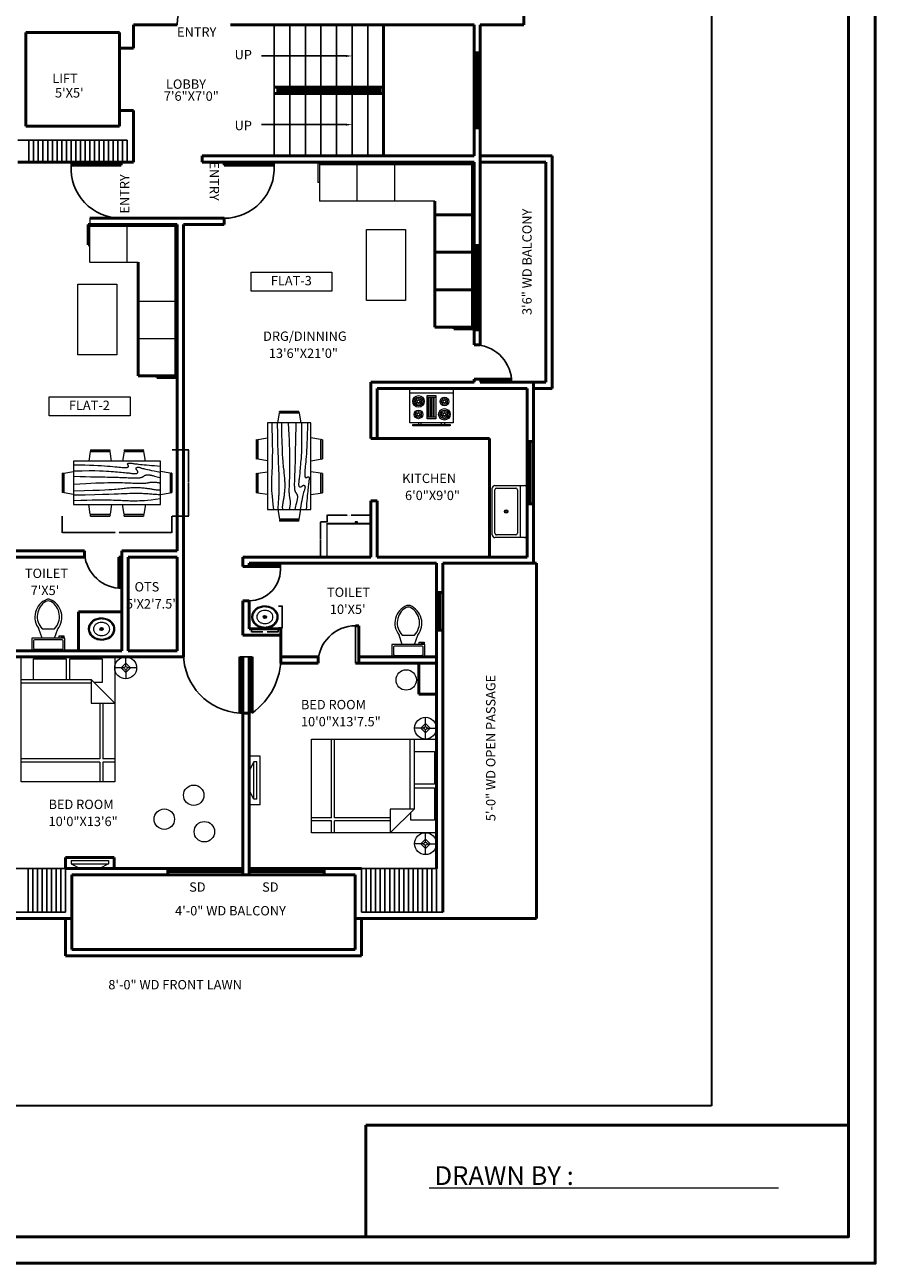
# Model space of a CAD drawing. Units: inches. Extents: x 1493 to 2377, y 814 to 2191.
# Tile 2 of 4: x 1832 to 2377, y 814 to 1607. Entities that reach past the tile are written whole.
import ezdxf
from ezdxf import colors
from ezdxf.entities.mleader import LeaderData, LeaderLine
from ezdxf.math import Vec2, Vec3

# ---------------------------------------------------------------- set-up
doc = ezdxf.new("R2010")
doc.units = ezdxf.units.IN
for name, color, linetype, lineweight in [('A-ANNO-DIMS', 2, 'Continuous', 18), ('A-ANNO-SYMB', 2, 'Continuous', 18), ('A-ANNO-TEXT', 3, 'Continuous', 18), ('A-ANNO-TTLB', 7, 'Continuous', 35), ('A-AREA-IDEN', 7, 'Continuous', 18), ('A-DOOR', 4, 'Continuous', 25), ('A-EQPM', 9, 'Continuous', 18), ('A-FLOR-FIXT', 8, 'Continuous', 18), ('A-FLOR-STRS', 3, 'Continuous', 25), ('A-FURN', 8, 'Continuous', 18), ('A-GLAZ', 4, 'Continuous', 25), ('A-WALL', 7, 'Continuous', 50)]:
    doc.layers.add(name, color=color, linetype=linetype, lineweight=lineweight)
doc.styles.get("Standard").update_dxf_attribs({"font": 'arial.ttf'})
doc.dimstyles.get("Standard").update_dxf_attribs({"dimtxt": 0.18, "dimasz": 0.18, "dimexe": 0.18, "dimexo": 0.0625, "dimgap": 0.09, "dimtad": 0, "dimtih": 1, "dimtoh": 1, "dimdec": 4, "dimzin": 0, "dimdsep": 46, "dimtxsty": 'Standard', "dimcen": 0.09, "dimadec": 0, "dimazin": 0, "dimtfac": 1, "dimtdec": 4, "dimtofl": 0, "dimtmove": 0, "dimatfit": 3, "dimfxl": 1, "dimtolj": 1, "dimtzin": 0, "dimarcsym": 0})

# ---------------------------------------------------------------- blocks, each defined once
blk = doc.blocks.new('Dining Set - 36 x 72 in.')
for p, q in [((-22.2343, 26.00059), (-23.4847, 17.99762)), ((-22.2304, 26), (-5.7608, 26)), ((-22, 27.5), (-22.1562, 26.50042)), ((-5.8416, 26.5), (-22.1534, 26.5)), ((-22, 27.5), (-6, 27.5)), ((-5.8437, 26.49966), (-6, 27.5)), ((-4.5152, 17.99762), (-5.7655, 25.99926)), ((5.7657, 26.00059), (4.5153, 17.99762)), ((5.7696, 26), (22.2392, 26)), ((6, 27.5), (5.8438, 26.50042)), ((22.1584, 26.5), (5.8466, 26.5)), ((6, 27.5), (22, 27.5)), ((22.1563, 26.49966), (22, 27.5)), ((23.4848, 17.99762), (22.2345, 25.99926)), ((36, 18), (-36, 18)), ((-36, 18), (-36, -18)), ((36, -18), (36, 18)), ((-45.5, 8), (-44.5004, 8.15617)), ((-45.5, 8), (-45.5, -8)), ((-44.5, -8.15843), (-44.5, 8.15338)), ((-44.0006, 8.23428), (-35.9976, 9.48474)), ((-44, 8.23041), (-44, -8.23915)), ((44.0006, 8.23428), (35.9976, 9.48474)), ((44, 8.23041), (44, -8.23915)), ((44.5, -8.15843), (44.5, 8.15338)), ((45.5, 8), (44.5005, 8.15617)), ((45.5, 8), (45.5, -8)), ((-44.4997, -8.15631), (-45.5, -8)), ((-35.9976, -9.48476), (-43.9993, -8.2345)), ((35.9976, -9.48476), (43.9993, -8.2345)), ((44.4997, -8.15631), (45.5, -8)), ((-36, -18), (36, -18)), ((-22.2343, -26.0006), (-23.4847, -17.99762)), ((-4.5152, -17.99762), (-5.7655, -25.99928)), ((5.7657, -26.0006), (4.5153, -17.99762)), ((23.4848, -17.99762), (22.2345, -25.99928)), ((-22.2304, -26), (-5.7608, -26)), ((-22, -27.5), (-22.1562, -26.50044)), ((-5.8416, -26.5), (-22.1534, -26.5)), ((-22, -27.5), (-6, -27.5)), ((-5.8437, -26.49967), (-6, -27.5)), ((5.7696, -26), (22.2392, -26)), ((6, -27.5), (5.8438, -26.50044)), ((22.1584, -26.5), (5.8466, -26.5)), ((6, -27.5), (22, -27.5)), ((22.1563, -26.49967), (22, -27.5))]:
    blk.add_line(p, q)
for points in [[(-36, 15), (-31.1772, 14.97754), (-26.8079, 14.91406), (-22.8538, 14.81543), (-19.276, 14.6875), (-16.0362, 14.53613), (-13.0957, 14.36718), (-10.4159, 14.18652), (-7.9583, 14), (-5.6904, 13.81315), (-3.6035, 13.63021), (-1.6954, 13.45508), (0.0365, 13.29166), (1.5945, 13.14388), (2.9811, 13.01562), (4.1988, 12.9108), (5.25, 12.83333), (6.1393, 12.78613), (6.8802, 12.76823), (7.4883, 12.77767), (7.9792, 12.8125), (8.3685, 12.87077), (8.6719, 12.95052), (8.9049, 13.0498), (9.0833, 13.16666), (9.2205, 13.29899), (9.3216, 13.44401), (9.3895, 13.59879), (9.4271, 13.76041), (9.4373, 13.92594), (9.4232, 14.09245), (9.3875, 14.257), (9.3333, 14.41666), (9.2638, 14.56917), (9.1836, 14.71484), (9.0975, 14.85465), (9.0104, 14.98958), (8.9272, 15.1206), (8.8529, 15.2487), (8.7922, 15.37483), (8.75, 15.5), (8.7305, 15.62467), (8.7344, 15.74739), (8.7617, 15.86621), (8.8125, 15.97916), (8.8867, 16.08431), (8.9844, 16.17968), (9.1055, 16.26334), (9.25, 16.33333), (9.4189, 16.38802), (9.6172, 16.42708), (9.8506, 16.45052), (10.125, 16.45833), (10.4463, 16.45052), (10.8203, 16.42708), (11.2529, 16.38802), (11.75, 16.33333), (12.3184, 16.26318), (12.9694, 16.17838), (13.7151, 16.07991), (14.5677, 15.96875), (15.5395, 15.84586), (16.6426, 15.71224), (17.8893, 15.56884), (19.2917, 15.41666), (20.859, 15.25667), (22.5879, 15.08984), (24.4721, 14.91715), (26.5052, 14.73958), (28.6809, 14.5581), (30.9929, 14.3737), (33.4347, 14.18733), (36, 14)], [(-36, 10), (-28.9766, 10.14274), (-23.1725, 10.20442), (-18.4241, 10.19775), (-14.5677, 10.13541), (-11.4399, 10.03011), (-8.877, 9.89453), (-6.7154, 9.74137), (-4.7917, 9.58333), (-2.9698, 9.43082), (-1.2246, 9.28515), (0.4415, 9.14534), (2.026, 9.01041), (3.5266, 8.87939), (4.9408, 8.7513), (6.266, 8.62516), (7.5, 8.5), (8.6411, 8.37549), (9.6914, 8.2539), (10.6538, 8.13818), (11.5312, 8.03125), (12.3267, 7.93603), (13.043, 7.85547), (13.6831, 7.79248), (14.25, 7.75), (14.7471, 7.7303), (15.1797, 7.73307), (15.5537, 7.75732), (15.875, 7.80208), (16.1494, 7.86637), (16.3828, 7.94922), (16.5811, 8.04964), (16.75, 8.16666), (16.8944, 8.29915), (17.0143, 8.44531), (17.1089, 8.60319), (17.1771, 8.77083), (17.218, 8.94629), (17.2305, 9.1276), (17.2137, 9.31282), (17.1667, 9.5), (17.0895, 9.6875), (16.987, 9.875), (16.8649, 10.0625), (16.7292, 10.25), (16.5856, 10.4375), (16.4401, 10.625), (16.2985, 10.8125), (16.1667, 11), (16.05, 11.18733), (15.9518, 11.3737), (15.8752, 11.5581), (15.8229, 11.73958), (15.798, 11.91715), (15.8034, 12.08984), (15.842, 12.25667), (15.9167, 12.41666), (16.0295, 12.56836), (16.1784, 12.70833), (16.3605, 12.83268), (16.5729, 12.9375), (16.8127, 13.01888), (17.0768, 13.07291), (17.3625, 13.0957), (17.6667, 13.08333), (17.9894, 13.03312), (18.3418, 12.94726), (18.7382, 12.82918), (19.1927, 12.68229), (19.7195, 12.51001), (20.3327, 12.31575), (21.0465, 12.10294), (21.875, 11.875), (22.8357, 11.63354), (23.959, 11.37304), (25.2786, 11.08618), (26.8282, 10.76562), (28.6414, 10.40405), (30.752, 9.99414), (33.1936, 9.52856), (36, 9)], [(-36, 5.5), (-30.7157, 5.3348), (-26.069, 5.20963), (-21.9946, 5.11767), (-18.4271, 5.05208), (-15.3009, 5.00602), (-12.5508, 4.97265), (-10.1112, 4.94515), (-7.9167, 4.91666), (-5.909, 4.88167), (-4.0586, 4.83984), (-2.3429, 4.79215), (-0.7396, 4.73958), (0.7739, 4.6831), (2.22, 4.6237), (3.6213, 4.56233), (5, 4.5), (6.373, 4.43782), (7.7344, 4.3776), (9.0723, 4.32129), (10.375, 4.27083), (11.6309, 4.22819), (12.8281, 4.19531), (13.9551, 4.17415), (15, 4.16666), (15.954, 4.17448), (16.819, 4.19791), (17.6001, 4.23698), (18.3021, 4.29166), (18.9299, 4.36198), (19.4883, 4.44791), (19.9823, 4.54948), (20.4167, 4.66666), (20.7969, 4.79899), (21.1302, 4.94401), (21.4245, 5.09879), (21.6875, 5.26041), (21.9271, 5.42594), (22.1511, 5.59245), (22.3672, 5.757), (22.5834, 5.91666), (22.8065, 6.06868), (23.0404, 6.21093), (23.2879, 6.34147), (23.5521, 6.45833), (23.8358, 6.55957), (24.142, 6.64323), (24.4735, 6.70735), (24.8334, 6.75), (25.2235, 6.76969), (25.642, 6.76692), (26.0858, 6.74267), (26.5521, 6.69791), (27.0379, 6.63362), (27.5404, 6.55078), (28.0565, 6.45036), (28.5834, 6.33333), (29.1242, 6.19987), (29.7071, 6.04687), (30.3661, 5.87044), (31.1354, 5.66666), (32.0493, 5.43164), (33.142, 5.16146), (34.4475, 4.85221), (36, 4.5)], [(-36, -1), (-30.7915, -0.6591), (-26.0195, -0.38216), (-21.6519, -0.16284), (-17.6563, 0.00521), (-14.0005, 0.12833), (-10.6523, 0.21289), (-7.5796, 0.26522), (-4.75, 0.29166), (-2.134, 0.29793), (0.2878, 0.28711), (2.5317, 0.26163), (4.6146, 0.22396), (6.5529, 0.17651), (8.3633, 0.12174), (10.0623, 0.06209), (11.6667, 0), (13.1899, -0.06201), (14.6341, -0.1211), (15.9982, -0.17432), (17.2813, -0.21875), (18.4823, -0.25147), (19.6003, -0.26953), (20.6343, -0.27002), (21.5834, -0.25), (22.4481, -0.20768), (23.2357, -0.14584), (23.9549, -0.06836), (24.6146, 0.02083), (25.2235, 0.11784), (25.7904, 0.21875), (26.3241, 0.31966), (26.8334, 0.41666), (27.3265, 0.50618), (27.8099, 0.58593), (28.2894, 0.65397), (28.7709, 0.70833), (29.2601, 0.74707), (29.763, 0.76823), (30.2855, 0.76985), (30.8334, 0.75), (31.4088, 0.70784), (31.9994, 0.64713), (32.589, 0.57275), (33.1615, 0.48958), (33.7008, 0.4025), (34.1908, 0.3164), (34.6153, 0.23616), (34.9584, 0.16666), (35.2099, 0.11165), (35.3848, 0.07031), (35.504, 0.04069), (35.5886, 0.02083), (35.6594, 0.00879), (35.7377, 0.0026), (35.8442, 0.00032), (36, 0)], [(-36, -6.5), (-27.1843, -6.31267), (-20.084, -6.1263), (-14.469, -5.9419), (-10.1094, -5.76042), (-6.7752, -5.58285), (-4.2363, -5.41016), (-2.2629, -5.24333), (-0.625, -5.08334), (0.8708, -4.93099), (2.2715, -4.78646), (3.5872, -4.64974), (4.8281, -4.52084), (6.0046, -4.39974), (7.127, -4.28646), (8.2053, -4.18099), (9.25, -4.08334), (10.2705, -3.99382), (11.2734, -3.91407), (12.2647, -3.84603), (13.25, -3.79167), (14.2354, -3.75293), (15.2266, -3.73177), (16.2295, -3.73015), (17.25, -3.75), (18.2912, -3.79248), (19.3451, -3.85547), (20.4009, -3.93604), (21.4479, -4.03125), (22.4754, -4.13819), (23.4727, -4.25391), (24.4289, -4.37549), (25.3334, -4.5), (26.1785, -4.62492), (26.9694, -4.74935), (27.7145, -4.87281), (28.4219, -4.99479), (29.1, -5.11483), (29.7572, -5.23242), (30.4016, -5.34709), (31.0417, -5.45834), (31.6837, -5.56437), (32.3262, -5.65821), (32.9658, -5.73153), (33.599, -5.77604), (34.2224, -5.78345), (34.8327, -5.74545), (35.4264, -5.65373), (36, -5.5)], [(-36, -10), (-26.4022, -9.81299), (-18.4675, -9.62891), (-11.9839, -9.45069), (-6.7396, -9.28125), (-2.5226, -9.12354), (0.8789, -8.98047), (3.6769, -8.85498), (6.0833, -8.75), (8.2767, -8.66765), (10.3021, -8.60677), (12.1712, -8.56543), (13.8958, -8.54167), (15.4876, -8.53353), (16.9583, -8.53907), (18.3197, -8.55632), (19.5834, -8.58334), (20.7616, -8.61841), (21.8685, -8.66081), (22.9188, -8.71004), (23.9271, -8.76563), (24.9081, -8.82707), (25.8763, -8.89388), (26.8465, -8.96558), (27.8334, -9.04167), (28.8474, -9.12118), (29.8828, -9.20117), (30.93, -9.27824), (31.9792, -9.34896), (33.0205, -9.40991), (34.0443, -9.45768), (35.0407, -9.48885), (36, -9.5)], [(-36, -14.5), (-30.0881, -14.33513), (-25.0332, -14.21224), (-20.7312, -14.12647), (-17.0781, -14.07292), (-13.97, -14.04671), (-11.3027, -14.04297), (-8.9724, -14.05681), (-6.875, -14.08334), (-4.9224, -14.11833), (-3.0905, -14.16016), (-1.3709, -14.20785), (0.2448, -14.26042), (1.7647, -14.3169), (3.1973, -14.3763), (4.5507, -14.43767), (5.8333, -14.5), (7.0554, -14.5621), (8.235, -14.62175), (9.3922, -14.67652), (10.5469, -14.72396), (11.7192, -14.76164), (12.929, -14.78711), (14.1965, -14.79794), (15.5417, -14.79167), (16.9933, -14.76424), (18.6152, -14.70508), (20.4804, -14.60197), (22.6615, -14.44271), (25.2312, -14.21509), (28.2624, -13.9069), (31.8277, -13.50594), (36, -13)]]:
    blk.add_lwpolyline(points)
blk = doc.blocks.new('Sink - Oval top')
for p, q in [((-1, 0), (1, 0)), ((0, 1), (0, -1))]:
    blk.add_line(p, q)
for points in [[(-12.2, 0.4, 0.117634), (-11.5, -3.4, 0.104469), (-8.9, -6.8, 0.090016), (-5.1, -9.1, 0.08192), (-0.3, -10, 0.08192), (4.5, -9.4, 0.090016), (8.4, -7.4, 0.104469), (11.2, -4.1, 0.117634), (12.2, -0.4, 0.117634), (11.5, 3.4, 0.104469), (8.9, 6.8, 0.090016), (5.1, 9.1, 0.08192), (0.3, 10, 0.08192), (-4.5, 9.4, 0.090016), (-8.4, 7.4, 0.104469), (-11.2, 4.1, 0.117634)], [(-11.3, 0.2, 0.118622), (-10.5, -3.3, 0.104678), (-8.1, -6.4, 0.089562), (-4.5, -8.4, 0.081185), (-0.1, -9.2, 0.081185), (4.3, -8.5, 0.089562), (7.9, -6.6, 0.104678), (10.4, -3.5, 0.118622), (11.3, -0.2, 0.118622), (10.5, 3.3, 0.104678), (8.1, 6.4, 0.089562), (4.5, 8.4, 0.081185), (0.1, 9.2, 0.081185), (-4.3, 8.5, 0.089562), (-7.9, 6.6, 0.104678), (-10.4, 3.5, 0.118622)], [(-7.4, 0.1, 0.118283), (-6.9, -2.2, 0.104607), (-5.3, -4.2, 0.089718), (-3, -5.5, 0.081436), (-0.1, -6, 0.081436), (2.8, -5.6, 0.089718), (5.2, -4.3, 0.104607), (6.9, -2.3, 0.118283), (7.4, -0.1, 0.118283), (6.9, 2.2, 0.104607), (5.3, 4.2, 0.089718), (3, 5.5, 0.081436), (0.1, 6, 0.081436), (-2.8, 5.6, 0.089718), (-5.2, 4.3, 0.104607), (-6.9, 2.3, 0.118283)]]:
    blk.add_lwpolyline(points, format="xyb", close=True)
for radius in [1.5, 1]:
    blk.add_circle((0, 0), radius)
blk = doc.blocks.new('Toilet - top')
for p, q in [((9.5, -6), (9.5, -2)), ((-10, -8.5), (-8, -8.5)), ((-10, -9.5), (-10, -8.5)), ((-7, -9.5), (-10, -9.5)), ((-8, -8.5), (-8, -8)), ((-7, -8), (-7, -9.5)), ((-4, -8), (-6, -14)), ((4, -14), (-4, -14)), ((4, -8), (6, -14))]:
    blk.add_line(p, q)
blk.add_lwpolyline([(10.5, -8), (10.5, 0), (-10.5, 0), (-10.5, -8)], close=True)
for points in [[(-9.5, -2), (-9.5, -6)], [(8.5, -1), (-8.5, -1)], [(-8.5, -7), (8.5, -7)]]:
    blk.add_lwpolyline(points)
for centre, radius, start, end in [((-8.62, -1.88), 0.884, 81.8699, 188.1301), ((-8.62, -6.12), 0.884, 171.8699, 278.1301), ((8.62, -1.88), 0.884, 351.8699, 98.1301), ((8.62, -6.12), 0.884, 261.8699, 8.1301), ((3.52, -21.58), 12.17, 141.46911, 247.97143), ((4.2, -21.82), 11.33, 136.36773, 238.94682), ((-3.52, -21.58), 12.17, 292.02843, 38.53071), ((-4.2, -21.82), 11.33, 301.05301, 43.63209), ((0, -27.88), 4, 245.73182, 294.26817), ((0, -29), 4, 254.86053, 285.13947)]:
    blk.add_arc(centre, radius, start, end)
blk = doc.blocks.new('Lamp - Table')
for p, q in [((-1, 0), (-7, 0)), ((0, 3), (-3, 0)), ((-3, 0), (0, -3)), ((0, 7), (0, 1)), ((3, 0), (0, 3)), ((0, -3), (3, 0)), ((1, 0), (7, 0)), ((0, -1), (0, -7))]:
    blk.add_line(p, q)
for radius in [7, 1]:
    blk.add_circle((0, 0), radius)
blk = doc.blocks.new('Bed - Queen')
for p, q in [((0, -80), (0, 0)), ((0, 0), (60, 0)), ((60, 0), (60, -80)), ((8, -1.2), (28.8, -1.2)), ((8, -14.4), (8, -1.2)), ((28.8, -1.2), (28.8, -14.4)), ((31.2, -1.2), (52, -1.2)), ((31.2, -14.4), (31.2, -1.2)), ((52, -1.2), (52, -16.4)), ((0, -14.4), (44.8, -14.4)), ((60, -29.6), (44.8, -14.4)), ((44.8, -14.4), (44.8, -29.6)), ((44.8, -16.8), (0, -16.8)), ((52, -16.4), (46.8, -16.4)), ((44.8, -29.6), (60, -29.6)), ((50.4, -29.6), (50.4, -65.35)), ((52.4, -29.6), (52.4, -65.35)), ((50.4, -65.35), (0, -65.35)), ((50.4, -67.35), (0, -67.35)), ((50.4, -67.35), (50.4, -80)), ((60, -65.35), (52.4, -65.35)), ((60, -67.35), (52.4, -67.35)), ((52.4, -67.35), (52.4, -80)), ((60, -80), (0, -80))]:
    blk.add_line(p, q)
blk = doc.blocks.new('Range-Oven - 30 in top')
for p, q in [((0, -3), (30, -3)), ((12, -6), (18, -6)), ((13, -20), (13, -6)), ((14, -6), (14, -20)), ((15, -20), (15, -6)), ((16, -6), (16, -20)), ((17, -20), (17, -6)), ((6, -24), (6, -25)), ((8, -25), (8, -24)), ((18, -20), (12, -20)), ((22, -25), (22, -24)), ((24, -24), (24, -25))]:
    blk.add_line(p, q)
for points in [[(0, -24), (0, 0), (30, 0), (30, -24)], [(12, -21), (12, -5), (18, -5), (18, -21)], [(2, -26), (2, -25), (28, -25), (28, -26)]]:
    blk.add_lwpolyline(points, close=True)
for centre, radius in [((6, -9), 4), ((6, -9), 3), ((6, -9), 2), ((6, -9), 1), ((24, -9), 3), ((24, -9), 2), ((24, -9), 1), ((6, -18), 3), ((6, -18), 2), ((6, -18), 1), ((24, -18), 4), ((24, -18), 3), ((24, -18), 2), ((24, -18), 1)]:
    blk.add_circle(centre, radius)
blk = doc.blocks.new('Sink-single - 30 in top')
blk.add_line((-15, -3.999996), (15, -3.999996))
for points in [[(-13.5, 0), (13.5, 0)], [(-15, -18.499996), (-15, -1.5)], [(-13.5, -17.499996), (-13.5, -6.499996)], [(-12.5, -5.499996), (12.5, -5.499996)], [(13.5, -6.499996), (13.5, -17.499996)], [(15, -1.5), (15, -18.499996)], [(13.5, -19.999996), (-13.5, -19.999996)], [(12.5, -18.499996), (-12.5, -18.499996)]]:
    blk.add_lwpolyline(points)
for radius in [1, 0.5]:
    blk.add_circle((0, -11.999996), radius)
for centre, radius, start, end in [((-13.5, -1.5), 1.5, 90, 180), ((-12.5, -6.499996), 1, 90, 180), ((12.5, -6.499996), 1, 0, 90), ((13.5, -1.5), 1.5, 0, 90), ((-13.5, -18.499996), 1.5, 180, 270), ((-12.5, -17.499996), 1, 180, 270), ((12.5, -17.499996), 1, 270, 0), ((13.5, -18.499996), 1.5, 270, 0)]:
    blk.add_arc(centre, radius, start, end)
blk = doc.blocks.new('Refrigerator-2 door - 36 in top')
for p, q in [((0, -26.999999), (36, -26.999999)), ((11, -27.999999), (11, -28.999999)), ((11, -28.999999), (13, -28.999999)), ((12, -26.999999), (12, -28.999999)), ((13, -28.999999), (13, -27.999999))]:
    blk.add_line(p, q)
blk.add_lwpolyline([(0, -27.999999), (0, 0), (36, 0), (36, -27.999999)], close=True)
blk = doc.blocks.new('AC-SPLIT-UNIT')
for p, q in [((-2, 27.5), (-2, -3.65)), ((-2, 27.5), (5, 27.5)), ((0, 24), (2, 24)), ((0, 24), (0, 0)), ((2, 24), (2, 0)), ((2, 24), (5, 18.22)), ((2, 0), (5, 5.78)), ((-2, -3.65), (5, -3.65)), ((0, 0), (2, 0))]:
    blk.add_line(p, q)
blk = doc.blocks.new('AC-INDOOR-UNIT')
for p, q in [((0, 0), (0, 24)), ((0, 24), (2, 24)), ((2, 0), (2, 24)), ((2, 24), (5, 18.22)), ((2, 0), (5, 5.78)), ((0, 0), (2, 0))]:
    blk.add_line(p, q)
blk = doc.blocks.new('*D20')
at = {"layer": 'A-ANNO-DIMS', "color": 0, "lineweight": -2, "transparency": 16777216}
for p, q in [((1977.36, 1220.86), (1977.36, 1218.17)), ((1977.54, 1218.35), (1984.58, 1218.35)), ((1994.33, 1218.35), (1987.29, 1218.35)), ((1994.51, 1220.86), (1994.51, 1218.17))]:
    blk.add_line(p, q, dxfattribs=at)
at = {"layer": 'A-ANNO-DIMS', "color": 0, "transparency": 16777216}
for points in [[(1977.54, 1218.38), (1977.54, 1218.32), (1977.36, 1218.35)], [(1994.33, 1218.38), (1994.33, 1218.32), (1994.51, 1218.35)]]:
    blk.add_solid(points, dxfattribs=at)
at = {"layer": 'Defpoints', "color": 0, "transparency": 16777216}
for p in [(1977.36, 1220.92), (1994.51, 1220.92), (1994.51, 1218.35)]:
    blk.add_point(p, dxfattribs=at)
at = {"layer": 'A-ANNO-DIMS', "color": 0, "transparency": 16777216, "insert": (1985.94, 1218.35), "char_height": 0.18, "attachment_point": 5}
blk.add_mtext('\\A1;WASH BASIN 17 TYP.', dxfattribs=at)
blk = doc.blocks.new('*D21')
at = {"layer": 'A-ANNO-DIMS', "color": 0, "lineweight": -2, "transparency": 16777216}
for p, q in [((1994.58, 1234.99), (1997.27, 1234.99)), ((1997.09, 1234.81), (1997.09, 1228.14)), ((1997.09, 1221.1), (1997.09, 1227.78)), ((1994.58, 1220.92), (1997.27, 1220.92))]:
    blk.add_line(p, q, dxfattribs=at)
at = {"layer": 'A-ANNO-DIMS', "color": 0, "transparency": 16777216}
for points in [[(1997.06, 1234.81), (1997.12, 1234.81), (1997.09, 1234.99)], [(1997.06, 1221.1), (1997.12, 1221.1), (1997.09, 1220.92)]]:
    blk.add_solid(points, dxfattribs=at)
at = {"layer": 'Defpoints', "color": 0, "transparency": 16777216}
for p in [(1994.51, 1234.99), (1997.09, 1234.99), (1994.51, 1220.92)]:
    blk.add_point(p, dxfattribs=at)
at = {"layer": 'A-ANNO-DIMS', "color": 0, "transparency": 16777216, "insert": (1997.09, 1227.96), "char_height": 0.18, "attachment_point": 5}
blk.add_mtext('\\A1;14 TYP.', dxfattribs=at)
blk = doc.blocks.new('*D32')
at = {"layer": 'A-ANNO-DIMS', "color": 0, "lineweight": -2, "transparency": 16777216}
for p, q in [((1856.13, 1292.54), (1856.13, 1281.88)), ((1926.41, 1292.54), (1926.41, 1281.88)), ((1856.31, 1282.06), (1889.99, 1282.06)), ((1926.23, 1282.06), (1892.55, 1282.06))]:
    blk.add_line(p, q, dxfattribs=at)
at = {"layer": 'A-ANNO-DIMS', "color": 0, "transparency": 16777216}
for points in [[(1856.31, 1282.09), (1856.31, 1282.03), (1856.13, 1282.06)], [(1926.23, 1282.09), (1926.23, 1282.03), (1926.41, 1282.06)]]:
    blk.add_solid(points, dxfattribs=at)
at = {"layer": 'Defpoints', "color": 0, "transparency": 16777216}
for p in [(1856.13, 1292.6), (1926.41, 1292.6), (1926.41, 1282.06)]:
    blk.add_point(p, dxfattribs=at)
at = {"layer": 'A-ANNO-DIMS', "color": 0, "transparency": 16777216, "insert": (1891.27, 1282.06), "char_height": 0.18, "attachment_point": 5}
blk.add_mtext('\\A1;DINING SET 70 TYP.', dxfattribs=at)
blk = doc.blocks.new('*D33')
at = {"layer": 'A-ANNO-DIMS', "color": 0, "lineweight": -2, "transparency": 16777216}
for p, q in [((1926.47, 1335.08), (1937.13, 1335.08)), ((1936.95, 1334.9), (1936.95, 1314.02)), ((1936.95, 1292.78), (1936.95, 1313.66)), ((1926.47, 1292.6), (1937.13, 1292.6))]:
    blk.add_line(p, q, dxfattribs=at)
at = {"layer": 'A-ANNO-DIMS', "color": 0, "transparency": 16777216}
for points in [[(1936.92, 1334.9), (1936.98, 1334.9), (1936.95, 1335.08)], [(1936.92, 1292.78), (1936.98, 1292.78), (1936.95, 1292.6)]]:
    blk.add_solid(points, dxfattribs=at)
at = {"layer": 'Defpoints', "color": 0, "transparency": 16777216}
for p in [(1926.41, 1335.08), (1936.95, 1335.08), (1926.41, 1292.6)]:
    blk.add_point(p, dxfattribs=at)
at = {"layer": 'A-ANNO-DIMS', "color": 0, "transparency": 16777216, "insert": (1936.95, 1313.84), "char_height": 0.18, "attachment_point": 5}
blk.add_mtext('\\A1;42 TYP.', dxfattribs=at)
blk = doc.blocks.new('*D36')
at = {"layer": 'A-ANNO-DIMS', "color": 0, "lineweight": -2, "transparency": 16777216}
for p, q in [((2025.83, 1288.99), (2025.83, 1293.3)), ((2053.83, 1288.99), (2053.83, 1293.3)), ((2026.01, 1293.12), (2038.58, 1293.12)), ((2053.65, 1293.12), (2041.08, 1293.12))]:
    blk.add_line(p, q, dxfattribs=at)
at = {"layer": 'A-ANNO-DIMS', "color": 0, "transparency": 16777216}
for points in [[(2026.01, 1293.15), (2026.01, 1293.09), (2025.83, 1293.12)], [(2053.65, 1293.15), (2053.65, 1293.09), (2053.83, 1293.12)]]:
    blk.add_solid(points, dxfattribs=at)
at = {"layer": 'Defpoints', "color": 0, "transparency": 16777216}
for p in [(2025.83, 1293.12), (2025.83, 1288.92), (2053.83, 1288.92)]:
    blk.add_point(p, dxfattribs=at)
at = {"layer": 'A-ANNO-DIMS', "color": 0, "transparency": 16777216, "insert": (2039.83, 1293.12), "char_height": 0.18, "attachment_point": 5}
blk.add_mtext('\\A1;REFRIGERATOR 28', dxfattribs=at)
blk = doc.blocks.new('*D37')
at = {"layer": 'A-ANNO-DIMS', "color": 0, "lineweight": -2, "transparency": 16777216}
for p, q in [((2025.77, 1288.92), (2021.45, 1288.92)), ((2021.63, 1288.74), (2021.63, 1277.83)), ((2021.63, 1266.55), (2021.63, 1277.46)), ((2025.77, 1266.37), (2021.45, 1266.37))]:
    blk.add_line(p, q, dxfattribs=at)
at = {"layer": 'A-ANNO-DIMS', "color": 0, "transparency": 16777216}
for points in [[(2021.6, 1288.74), (2021.66, 1288.74), (2021.63, 1288.92)], [(2021.6, 1266.55), (2021.66, 1266.55), (2021.63, 1266.37)]]:
    blk.add_solid(points, dxfattribs=at)
at = {"layer": 'Defpoints', "color": 0, "transparency": 16777216}
for p in [(2025.83, 1288.92), (2021.63, 1266.37), (2025.83, 1266.37)]:
    blk.add_point(p, dxfattribs=at)
at = {"layer": 'A-ANNO-DIMS', "color": 0, "transparency": 16777216, "insert": (2021.63, 1277.64), "char_height": 0.18, "attachment_point": 5}
blk.add_mtext('\\A1;23', dxfattribs=at)

msp = doc.modelspace()

# ---------------------------------------------------------------- linework, layer by layer
at = {"layer": 'A-ANNO-SYMB'}
for points in [[(1977.18, 1448.82), (2028.87, 1448.82), (2028.87, 1436.73), (1977.18, 1436.73)], [(1847.86, 1368.94), (1899.55, 1368.94), (1899.55, 1356.85), (1847.86, 1356.85)]]:
    msp.add_lwpolyline(points, close=True, dxfattribs=at)
at = {"layer": 'A-ANNO-TEXT'}
msp.add_line((2091.09, 862.14), (2314.82, 862.14), dxfattribs=at)
at = {"layer": 'A-ANNO-TTLB'}
for p, q in [((2271.83, 2093.87), (2271.83, 914.87)), ((2271.83, 914.87), (1603.83, 914.87))]:
    msp.add_line(p, q, dxfattribs=at)
at = {"layer": 'A-DOOR'}
for p, q in [((1861.83, 1518.37), (1861.83, 1517.37)), ((1991.81, 1518.37), (1991.81, 1517.37)), ((2143.83, 1379.37), (2123.83, 1379.37)), ((2123.83, 1379.37), (2123.83, 1378.37)), ((2143.83, 1380.37), (2143.83, 1379.37)), ((1893.33, 1266.37), (1893.33, 1246.37)), ((1995.83, 1261.37), (1995.83, 1260.37)), ((1893.33, 1246.37), (1892.33, 1246.37)), ((2044.02, 1222.37), (2044.02, 1198.37)), ((1977.83, 1202.37), (1969.83, 1202.37)), ((1970.83, 1202.37), (1970.83, 1166.44)), ((1970.83, 1166.44), (1969.83, 1166.44))]:
    msp.add_line(p, q, dxfattribs=at)
for centre, radius, start, end in [((1965.89, 1607.37), 36.06, 93.27315, 180), ((1893.83, 1515.43), 32.06, 176.52859, 270), ((1959.81, 1515.43), 32.06, 270, 3.47141), ((2119.83, 1378.28), 24.09, 4.97911, 90), ((1894.42, 1270.37), 24.09, 180, 265.02089), ((1975.83, 1258.46), 20.09, 270, 5.45262), ((2044.02, 1198.37), 24, 90, 180), ((1971.89, 1204.44), 38.06, 180, 266.90368), ((1951.77, 1202.37), 44.44, 305.90347, 0)]:
    msp.add_arc(centre, radius, start, end, dxfattribs=at)
at = {"layer": 'A-FLOR-FIXT'}
msp.add_circle((2076.41, 1187.6), 6.53, dxfattribs=at)
at = {"layer": 'A-FLOR-STRS'}
for p, q in [((1991.83, 1607.37), (1991.83, 1523.37)), ((2001.83, 1607.37), (2001.83, 1567.37)), ((2011.83, 1607.37), (2011.83, 1567.37)), ((2021.83, 1607.37), (2021.83, 1567.37)), ((2031.83, 1607.37), (2031.83, 1567.37)), ((2041.83, 1607.37), (2041.83, 1567.37)), ((2051.83, 1607.37), (2051.83, 1567.37)), ((1993.83, 1566.37), (1993.83, 1564.37)), ((2001.83, 1563.37), (2001.83, 1523.37)), ((2011.83, 1563.37), (2011.83, 1523.37)), ((2021.83, 1563.37), (2021.83, 1523.37)), ((2031.83, 1563.37), (2031.83, 1523.37)), ((2041.83, 1563.37), (2041.83, 1523.37)), ((2051.83, 1563.37), (2051.83, 1523.37))]:
    msp.add_line(p, q, dxfattribs=at)
at = {"layer": 'A-FURN'}
for p, q in [((2019.83, 1519.37), (2019.83, 1506.37)), ((2020.83, 1518.37), (2020.83, 1494.37)), ((2044.83, 1518.37), (2044.83, 1494.37)), ((2068.83, 1518.37), (2068.83, 1494.37)), ((2020.83, 1506.37), (2019.83, 1506.37)), ((2070.83, 1494.37), (2020.83, 1494.37)), ((2094.83, 1494.37), (2020.83, 1494.37)), ((1873.83, 1483.37), (1873.83, 1479.37)), ((1873.83, 1478.37), (1928.83, 1478.37)), ((1873.83, 1455.37), (1873.83, 1478.37)), ((1901.83, 1483.37), (1897.83, 1483.37)), ((1897.83, 1455.37), (1897.83, 1478.37)), ((1873.83, 1455.37), (1904.83, 1455.37)), ((1904.83, 1430.37), (1928.83, 1430.37)), ((1904.83, 1406.37), (1928.83, 1406.37))]:
    msp.add_line(p, q, dxfattribs=at)
for points in [[(2050.98, 1476.21), (2075.98, 1476.21), (2075.98, 1430.79), (2050.98, 1430.79)], [(1866.06, 1441.25), (1891.06, 1441.25), (1891.06, 1395.83), (1866.06, 1395.83)]]:
    msp.add_lwpolyline(points, close=True, dxfattribs=at)
for centre in [(1940.34, 1113.75), (1921.52, 1098.44), (1947.17, 1090.4)]:
    msp.add_circle(centre, 6.53, dxfattribs=at)
at = {"layer": 'A-GLAZ'}
for p, q in [((1897.83, 1533.37), (1827.83, 1533.37)), ((1834.83, 1533.37), (1834.83, 1519.37)), ((1837.83, 1533.37), (1837.83, 1519.37)), ((1840.83, 1533.37), (1840.83, 1519.37)), ((1843.83, 1533.37), (1843.83, 1519.37)), ((1846.83, 1533.37), (1846.83, 1519.37)), ((1849.83, 1533.37), (1849.83, 1519.37)), ((1852.83, 1533.37), (1852.83, 1519.37)), ((1855.83, 1533.37), (1855.83, 1519.37)), ((1858.83, 1533.37), (1858.83, 1519.37)), ((1861.83, 1533.37), (1861.83, 1519.37)), ((1864.83, 1533.37), (1864.83, 1519.37)), ((1867.83, 1533.37), (1867.83, 1519.37)), ((1870.83, 1533.37), (1870.83, 1519.37)), ((1873.83, 1533.37), (1873.83, 1519.37)), ((1876.83, 1533.37), (1876.83, 1519.37)), ((1879.83, 1533.37), (1879.83, 1519.37)), ((1882.83, 1533.37), (1882.83, 1519.37)), ((1885.83, 1533.37), (1885.83, 1519.37)), ((1888.83, 1533.37), (1888.83, 1519.37)), ((1891.83, 1533.37), (1891.83, 1519.37)), ((1894.83, 1533.37), (1894.83, 1519.37)), ((1897.83, 1533.37), (1897.83, 1519.37)), ((1855.33, 1066.87), (1810.33, 1066.87)), ((1834.33, 1066.87), (1834.33, 1038.87)), ((1837.33, 1066.87), (1837.33, 1038.87)), ((1840.33, 1066.87), (1840.33, 1038.87)), ((1843.33, 1066.87), (1843.33, 1038.87)), ((1846.33, 1066.87), (1846.33, 1038.87)), ((1849.33, 1066.87), (1849.33, 1038.87)), ((1852.33, 1066.87), (1852.33, 1038.87)), ((1855.33, 1066.87), (1855.33, 1038.87)), ((1855.33, 1066.87), (1858.33, 1066.87)), ((1858.33, 1066.87), (1858.33, 1038.87)), ((2047.83, 1066.87), (2047.83, 1038.87)), ((2047.83, 1066.87), (2050.83, 1066.87)), ((2092.83, 1066.87), (2050.83, 1066.87)), ((2050.83, 1066.87), (2050.83, 1038.87)), ((2053.83, 1066.87), (2053.83, 1038.87)), ((2056.83, 1066.87), (2056.83, 1038.87)), ((2059.83, 1066.87), (2059.83, 1038.87)), ((2062.83, 1066.87), (2062.83, 1038.87)), ((2065.83, 1066.87), (2065.83, 1038.87)), ((2068.83, 1066.87), (2068.83, 1038.87)), ((2071.83, 1066.87), (2071.83, 1038.87)), ((2074.83, 1066.87), (2074.83, 1038.87)), ((2077.83, 1066.87), (2077.83, 1038.87)), ((2080.83, 1066.87), (2080.83, 1038.87)), ((2083.83, 1066.87), (2083.83, 1038.87)), ((2086.83, 1066.87), (2086.83, 1038.87)), ((2089.83, 1066.87), (2089.83, 1038.87)), ((2092.83, 1066.87), (2092.83, 1038.87)), ((2092.83, 1066.87), (2095.83, 1066.87)), ((2095.83, 1066.87), (2095.83, 1038.87)), ((1858.33, 1038.87), (1810.33, 1038.87)), ((2099.83, 1038.87), (2047.83, 1038.87))]:
    msp.add_line(p, q, dxfattribs=at)
at = {"layer": 'A-WALL'}
for p, q in [((2151.83, 1659.37), (2151.83, 1607.37)), ((1901.83, 1607.37), (1901.83, 1592.37)), ((1929.83, 1607.37), (1901.83, 1607.37)), ((2119.83, 1607.37), (1963.83, 1607.37)), ((2061.83, 1607.37), (2061.83, 1523.37)), ((2119.83, 1607.37), (2119.83, 1523.37)), ((2151.83, 1607.37), (2123.83, 1607.37)), ((2123.83, 1607.37), (2123.83, 1402.37)), ((1832.83, 1602.37), (1832.83, 1542.37)), ((1892.83, 1602.37), (1832.83, 1602.37)), ((1892.83, 1602.37), (1892.83, 1542.37)), ((1892.83, 1592.37), (1901.83, 1592.37)), ((2119.83, 1589.37), (2123.83, 1589.37)), ((2121.83, 1589.37), (2121.83, 1541.37)), ((2061.83, 1567.37), (1991.83, 1567.37)), ((2061.83, 1563.37), (1991.83, 1563.37)), ((2059.83, 1566.37), (1993.83, 1566.37)), ((2059.83, 1564.37), (1993.83, 1564.37)), ((2059.83, 1566.37), (2059.83, 1564.37)), ((1892.83, 1552.37), (1901.83, 1552.37)), ((1901.83, 1552.37), (1901.83, 1519.37)), ((1892.83, 1542.37), (1832.83, 1542.37)), ((2119.83, 1541.37), (2123.83, 1541.37)), ((1901.83, 1519.37), (1827.83, 1519.37)), ((1893.83, 1518.37), (1861.83, 1518.37)), ((1893.83, 1517.37), (1861.83, 1517.37)), ((1893.83, 1519.37), (1893.83, 1517.37)), ((1945.83, 1519.37), (1945.83, 1523.37)), ((2119.83, 1523.37), (1945.83, 1523.37)), ((2119.83, 1519.37), (1945.83, 1519.37)), ((1959.81, 1517.37), (1959.81, 1519.37)), ((1991.81, 1518.37), (1959.81, 1518.37)), ((1991.81, 1517.37), (1959.81, 1517.37)), ((2118.83, 1518.37), (2020.83, 1518.37)), ((2118.83, 1518.37), (2118.83, 1413.6)), ((2119.83, 1519.37), (2119.83, 1402.37)), ((2169.83, 1523.37), (2123.83, 1523.37)), ((2165.83, 1519.37), (2123.83, 1519.37)), ((2157.83, 1519.37), (2153.83, 1519.37)), ((2165.83, 1519.37), (2165.83, 1378.37)), ((2169.83, 1523.37), (2169.83, 1374.37)), ((2094.83, 1494.37), (2094.83, 1413.6)), ((2094.83, 1485.6), (2118.83, 1485.6)), ((1872.83, 1479.37), (1929.83, 1479.37)), ((1872.83, 1466.37), (1872.83, 1479.37)), ((1873.83, 1483.37), (1959.81, 1483.37)), ((1928.83, 1478.37), (1928.83, 1382.37)), ((1933.83, 1483.37), (1929.83, 1483.37)), ((1929.83, 1479.37), (1929.83, 1270.37)), ((1933.83, 1479.37), (1933.83, 1202.37)), ((1933.83, 1479.37), (1959.81, 1479.37)), ((1959.81, 1483.37), (1959.81, 1479.37)), ((1872.83, 1466.37), (1873.83, 1466.37)), ((2094.83, 1461.6), (2118.83, 1461.6)), ((2119.83, 1465.98), (2123.83, 1465.98)), ((2121.83, 1465.98), (2121.83, 1411.87)), ((1904.83, 1455.37), (1904.83, 1382.37)), ((2094.83, 1437.6), (2118.83, 1437.6)), ((2094.83, 1413.6), (2118.83, 1413.6)), ((2106.83, 1413.6), (2106.83, 1412.6)), ((2106.83, 1412.6), (2119.83, 1412.6)), ((2123.83, 1411.87), (2119.83, 1411.87)), ((2123.83, 1402.37), (2119.83, 1402.37)), ((1904.83, 1382.37), (1928.83, 1382.37)), ((1916.83, 1382.37), (1916.83, 1381.37)), ((1916.83, 1381.37), (1929.83, 1381.37)), ((2053.83, 1378.37), (2053.83, 1342.37)), ((2119.83, 1378.37), (2053.83, 1378.37)), ((2057.83, 1374.37), (2057.83, 1342.37)), ((2153.83, 1374.37), (2057.83, 1374.37)), ((2143.83, 1380.37), (2119.83, 1380.37)), ((2119.83, 1380.37), (2119.83, 1378.37)), ((2165.83, 1378.37), (2123.83, 1378.37)), ((2153.83, 1374.37), (2153.83, 1266.37)), ((2157.83, 1378.37), (2157.83, 1262.37)), ((2169.83, 1374.37), (2157.83, 1374.37)), ((2053.83, 1342.37), (2057.83, 1342.37)), ((2057.83, 1342.37), (2129.83, 1342.37)), ((2129.83, 1342.37), (2129.83, 1266.37)), ((2153.83, 1340.37), (2157.83, 1340.37)), ((2153.83, 1340.37), (2157.83, 1340.37)), ((2153.83, 1340.37), (2157.83, 1340.37)), ((2155.83, 1340.37), (2155.83, 1300.37)), ((2053.83, 1302.37), (2057.83, 1302.37)), ((2053.83, 1302.37), (2053.83, 1266.37)), ((2057.83, 1302.37), (2057.83, 1266.37)), ((2153.83, 1300.37), (2157.83, 1300.37)), ((1870.33, 1270.37), (1805.33, 1270.37)), ((1870.33, 1270.37), (1870.33, 1266.37)), ((1894.33, 1270.37), (1894.33, 1206.37)), ((1929.83, 1270.37), (1894.33, 1270.37)), ((1870.33, 1266.37), (1810.33, 1266.37)), ((1892.33, 1266.37), (1892.33, 1246.37)), ((1894.33, 1266.37), (1892.33, 1266.37)), ((1898.33, 1266.37), (1898.33, 1206.37)), ((1929.83, 1266.37), (1898.33, 1266.37)), ((1929.83, 1266.37), (1929.83, 1206.37)), ((1971.83, 1266.37), (1971.83, 1260.37)), ((2053.83, 1266.37), (1971.83, 1266.37)), ((2053.83, 1266.37), (1971.83, 1266.37)), ((1975.83, 1262.37), (1975.83, 1260.37)), ((2095.83, 1262.37), (1975.83, 1262.37)), ((2153.83, 1266.37), (2057.83, 1266.37)), ((2099.83, 1266.37), (2057.83, 1266.37)), ((2095.83, 1262.37), (2095.83, 1235.26)), ((2095.83, 1262.37), (2095.83, 1066.87)), ((2159.83, 1262.37), (2099.83, 1262.37)), ((2099.83, 1262.37), (2099.83, 1066.87)), ((2159.83, 1262.37), (2159.83, 1034.87)), ((1995.83, 1260.37), (1971.83, 1260.37)), ((1995.83, 1261.37), (1975.83, 1261.37)), ((1975.83, 1238.37), (1971.83, 1238.37)), ((1971.83, 1238.37), (1971.83, 1216.37)), ((1975.83, 1238.37), (1975.83, 1220.37)), ((2095.83, 1243.56), (2099.83, 1243.56)), ((2095.83, 1243.56), (2099.83, 1243.56)), ((2097.83, 1243.56), (2097.83, 1219.56)), ((1866.62, 1206.37), (1866.62, 1231.32)), ((1866.62, 1231.32), (1894.33, 1231.32)), ((2046.02, 1222.37), (2044.02, 1222.37)), ((2046.02, 1198.37), (2046.02, 1222.37)), ((1971.83, 1216.37), (1996.21, 1216.37)), ((1975.83, 1220.37), (1996.21, 1220.37)), ((1996.21, 1220.37), (1996.21, 1198.37)), ((2095.83, 1219.56), (2099.83, 1219.56)), ((1894.33, 1206.37), (1810.33, 1206.37)), ((1929.83, 1206.37), (1898.33, 1206.37)), ((1933.89, 1202.37), (1810.33, 1202.37)), ((1969.83, 1202.37), (1969.83, 1166.44)), ((1971.83, 1202.37), (1971.83, 1066.87)), ((1975.83, 1202.37), (1975.83, 1066.87)), ((1977.83, 1202.37), (1977.83, 1166.37)), ((2020.02, 1202.37), (1996.21, 1202.37)), ((2020.02, 1198.37), (1996.21, 1198.37)), ((2020.02, 1202.37), (2020.02, 1198.37)), ((2095.83, 1198.37), (2044.02, 1198.37)), ((2044.02, 1198.37), (2046.02, 1198.37)), ((2095.83, 1202.37), (2046.02, 1202.37)), ((2084.56, 1198.37), (2084.56, 1178.52)), ((2084.56, 1178.52), (2095.83, 1178.52)), ((1975.83, 1166.37), (1971.83, 1166.37)), ((1858.33, 1073.87), (1889.49, 1073.87)), ((1858.33, 1073.87), (1858.33, 1066.87)), ((1889.49, 1073.87), (1889.49, 1066.87)), ((1971.83, 1066.87), (1858.33, 1066.87)), ((1923.83, 1066.87), (1923.83, 1062.87)), ((1923.83, 1064.87), (1971.83, 1064.87)), ((1971.83, 1066.87), (1971.83, 1062.87)), ((1975.83, 1066.87), (1975.83, 1062.87)), ((2047.83, 1066.87), (1975.83, 1066.87)), ((2023.83, 1064.87), (1975.83, 1064.87)), ((2023.83, 1066.87), (2023.83, 1062.87)), ((2099.83, 1066.87), (2099.83, 1038.87)), ((2043.83, 1062.87), (1862.33, 1062.87)), ((1862.33, 1062.87), (1862.33, 1014.87)), ((2043.83, 1062.87), (2043.83, 1014.87)), ((1862.33, 1034.87), (1806.33, 1034.87)), ((1858.33, 1034.87), (1858.33, 1010.87)), ((2159.83, 1034.87), (2043.83, 1034.87)), ((2047.83, 1034.87), (2047.83, 1010.87)), ((2047.83, 1010.87), (1858.33, 1010.87)), ((1899.83, 1014.87), (1862.33, 1014.87)), ((2043.83, 1014.87), (1899.83, 1014.87)), ((2359.73, 902.32), (2050.59, 902.32)), ((2050.59, 902.32), (2050.59, 830.94))]:
    msp.add_line(p, q, dxfattribs=at)
for points in [[(1493.21, 2190.87), (2376.73, 2190.87), (2376.73, 813.94), (1493.21, 813.94)], [(1510.21, 2173.87), (2359.73, 2173.87), (2359.73, 830.94), (1510.21, 830.94)]]:
    msp.add_lwpolyline(points, close=True, dxfattribs=at)

# ---------------------------------------------------------------- block references
at = {"layer": 'A-EQPM', "xscale": 0.9223664776301376, "yscale": 0.9223664776301376, "zscale": 0.9223664776301376}
msp.add_blockref('Range-Oven - 30 in top', (2078.71, 1374.38), dxfattribs=at)
at = {"layer": 'A-EQPM', "xscale": 0.7777777500000033, "yscale": 0.7777777500000033, "zscale": 0.7777777500000033, "rotation": 180}
msp.add_blockref('Refrigerator-2 door - 36 in top', (2053.83, 1266.37), dxfattribs=at)
at = {"layer": 'A-EQPM'}
for name, p, rotation in [('AC-SPLIT-UNIT', (1980.81, 1135.19), 180.0844183609336), ('AC-INDOOR-UNIT', (1861.83, 1071.87), 269.9999999999988)]:
    msp.add_blockref(name, p, dxfattribs=dict(at, rotation=rotation))
at = {"layer": 'A-FLOR-FIXT', "xscale": 1.112314284845436, "yscale": 1.112314284845436, "zscale": 1.112314284845436, "rotation": 270}
msp.add_blockref('Sink-single - 30 in top', (2153.79, 1295.53), dxfattribs=at)
at = {"layer": 'A-FLOR-FIXT', "rotation": 180}
for p in [(1847.27, 1206.37), (2077.81, 1202.37)]:
    msp.add_blockref('Toilet - top', p, dxfattribs=at)
at = {"layer": 'A-FLOR-FIXT', "xscale": 0.6987235820386822, "yscale": 0.6987235820386822, "zscale": 0.6987235820386822}
for p in [(1985.94, 1227.96), (1881.37, 1220.25)]:
    msp.add_blockref('Sink - Oval top', p, dxfattribs=at)
at = {"layer": 'A-FURN', "xscale": 0.7723268077391945, "yscale": 0.7723268077391945, "zscale": 0.7723268077391945, "rotation": 270}
msp.add_blockref('Dining Set - 36 x 72 in.', (2001.54, 1324.54), dxfattribs=at)
at = {"layer": 'A-FURN', "xscale": 0.7723268077391945, "yscale": 0.7723268077391945, "zscale": 0.7723268077391945}
msp.add_blockref('Dining Set - 36 x 72 in.', (1891.27, 1313.84), dxfattribs=at)
at = {"layer": 'A-FURN'}
msp.add_blockref('Bed - Queen', (1829.79, 1202.37), dxfattribs=at)
for name, p, rotation in [('Lamp - Table', (1896.79, 1195.33), 270), ('Lamp - Table', (2088.8, 1156.71), 180), ('Bed - Queen', (2095.83, 1149.72), 270), ('Lamp - Table', (2088.8, 1082.72), 180)]:
    msp.add_blockref(name, p, dxfattribs=dict(at, rotation=rotation))

# ---------------------------------------------------------------- texts
at = {"layer": 'A-AREA-IDEN'}
for s, height, p in [('      ENTRY', 6, (1918.66, 1599.77)), ('              UP', 6, (1940.89, 1585.22)), ('         LIFT', 6, (1833.29, 1569.97)), ('      LOBBY', 6, (1911.57, 1566.35)), ("      5'X5'", 6, (1840.53, 1560.77)), ('  7\'6"X7\'0"', 6, (1917.57, 1558.65)), ('              UP', 6, (1940.89, 1539.84)), ('FLAT-3', 6, (1989.73, 1440.44)), ('DRG/DINNING', 6, (1984.78, 1404.85)), ('  13\'6"X21\'0"', 6, (1984.78, 1393.92)), ('FLAT-2', 6, (1860.42, 1360.57)), ('  KITCHEN', 6, (2070.17, 1313.78)), ('   6\'0"X9\'0"', 6, (2070.17, 1302.86)), ('TOILET', 6, (1832.26, 1252.92)), ("  7'X5'", 6, (1832.26, 1242)), ('      OTS', 6, (1891.45, 1244.3)), ('TOILET', 6, (2025.71, 1240.84)), ('   5\'X2\'7.5"', 6, (1891.45, 1233.38)), (" 10'X5'", 6, (2025.71, 1229.91)), ('BED ROOM', 6, (2009.02, 1168.82)), ('10\'0"X13\'7.5"', 6, (2009.02, 1157.9)), ('BED ROOM', 6, (1847.41, 1104.91)), ('10\'0"X13\'6"', 6, (1847.41, 1093.98)), ('      SD', 6, (1926.45, 1051.95)), ('      SD', 6, (1973.15, 1051.95)), ('4\'-0" WD BALCONY', 6, (1928.43, 1036.76)), ('8\'-0" WD FRONT LAWN', 6, (1885.68, 989.39)), ('DRAWN BY :', 12, (2094.57, 864.07))]:
    msp.add_text(s, height=height, dxfattribs=at).set_placement(p)
for s, rotation, p in [('      ENTRY', 270, (1950.62, 1530.85)), ('      ENTRY', 90, (1899.04, 1475.41)), ('3\'6" WD BALCONY', 90, (2156.75, 1421.43)), ('5\'-0" WD OPEN PASSAGE', 90, (2133.54, 1097.17))]:
    msp.add_text(s, height=6, rotation=rotation, dxfattribs=at).set_placement(p)

# ---------------------------------------------------------------- dimensions: what is measured, and where the dimension line sits
at = {"layer": 'A-ANNO-DIMS'}
for base, p1, p2, angle, text, picture, middle in [((1936.95, 1335.08), (1926.41, 1292.6), (1926.41, 1335.08), 90, '<> TYP.', '*D33', (1936.95, 1313.84)), ((2025.83, 1293.12), (2053.83, 1288.92), (2025.83, 1288.92), 180, 'REFRIGERATOR <>', '*D36', (2039.83, 1293.12)), ((1997.09, 1234.99), (1994.51, 1220.92), (1994.51, 1234.99), 90, '<> TYP.', '*D21', (1997.09, 1227.96))]:
    dim = msp.add_linear_dim(base=base, p1=p1, p2=p2, angle=angle, text=text, dimstyle='Standard', override={"dimdec": 0, "dimlfac": 1, "dimrnd": 0, "dimzin": 0, "dimdsep": 46, "dimlunit": 2}, dxfattribs=at)
    dim.commit()
    dim.dimension.update_dxf_attribs({"geometry": picture, "text_midpoint": middle})
for base, p1, p2, text, picture, middle in [((1926.41, 1282.06), (1856.13, 1292.6), (1926.41, 1292.6), 'DINING SET <> TYP.', '*D32', (1891.27, 1282.06)), ((1994.51, 1218.35), (1977.36, 1220.92), (1994.51, 1220.92), 'WASH BASIN <> TYP.', '*D20', (1985.94, 1218.35))]:
    dim = msp.add_linear_dim(base=base, p1=p1, p2=p2, text=text, dimstyle='Standard', override={"dimdec": 0, "dimlfac": 1, "dimrnd": 0, "dimzin": 0, "dimdsep": 46, "dimlunit": 2}, dxfattribs=at)
    dim.commit()
    dim.dimension.update_dxf_attribs({"geometry": picture, "text_midpoint": middle})
dim = msp.add_linear_dim(base=(2021.63, 1266.37), p1=(2025.83, 1288.92), p2=(2025.83, 1266.37), angle=270, dimstyle='Standard', override={"dimdec": 0, "dimlfac": 1, "dimrnd": 0, "dimzin": 0, "dimdsep": 46, "dimlunit": 2}, dxfattribs=at)
dim.commit()
dim.dimension.update_dxf_attribs({"geometry": '*D37', "text_midpoint": (2021.63, 1277.64)})

# ---------------------------------------------------------------- leaders
at = {"layer": 'A-ANNO-TEXT'}
ml = msp.add_multileader_mtext('Standard', dxfattribs=at)
ml.set_content('', color=256)
ml.set_leader_properties()
ml.build(insert=Vec2(0, 0))
ctx = ml.context
ctx.base_point, ctx.plane_origin, ctx.plane_x_axis, ctx.plane_y_axis = Vec3(1983.83, 1587.37), Vec3(2041.83, 1587.37), Vec3(-1, 0), Vec3(0, -1)
notes = []
notes.append((ctx, [(0, (1, 1, 0), (1991.83, 1587.37), (-1, 0), 8, [(0, [(2041.83, 1587.37)], 0, [])])]))
ctx.mtext.insert, ctx.mtext.text_direction, ctx.mtext.rotation, ctx.mtext.flow_direction = Vec3(1981.83, 1585.37), Vec3(-1, 0), 3.141593, 5
ml = msp.add_multileader_mtext('Standard', dxfattribs=at)
ml.set_content('', color=256)
ml.set_leader_properties()
ml.build(insert=Vec2(0, 0))
ctx = ml.context
ctx.base_point, ctx.plane_origin, ctx.plane_x_axis, ctx.plane_y_axis = Vec3(1983.83, 1543.37), Vec3(2041.83, 1543.37), Vec3(-1, 0), Vec3(0, -1)
notes.append((ctx, [(0, (1, 1, 0), (1991.83, 1543.37), (-1, 0), 8, [(0, [(2041.83, 1543.37)], 0, [])])]))
ctx.mtext.insert, ctx.mtext.text_direction, ctx.mtext.rotation, ctx.mtext.flow_direction = Vec3(1981.83, 1541.37), Vec3(-1, 0), 3.141593, 5
for ctx, leaders in notes:
    for number, flags, end, landing, length, lines in leaders:
        leader = LeaderData()
        leader.index, (leader.has_last_leader_line, leader.has_dogleg_vector, leader.attachment_direction) = number, flags
        leader.last_leader_point, leader.dogleg_vector, leader.dogleg_length = Vec3(end), Vec3(landing), length
        for number, points, colour, breaks in lines:
            line = LeaderLine()
            line.index, line.vertices, line.color, line.breaks = number, Vec3.list(points), colors.encode_raw_color(colour), breaks
            leader.lines.append(line)
        ctx.leaders.append(leader)

doc.saveas('drawing.dxf')
